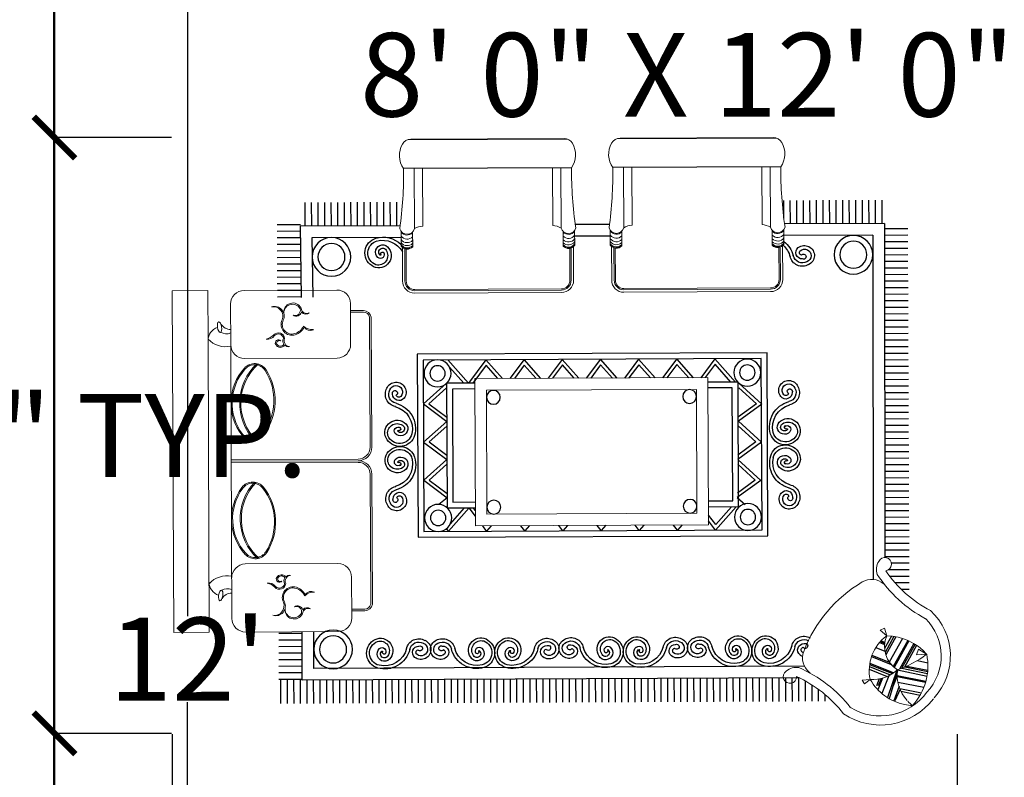
# Model space of a CAD drawing. Units: inches. Extents: x 147 to 1638, y 107 to 941.
# Tile 6 of 17: x 469 to 541, y 315 to 370. Entities that reach past the tile are written whole.
import ezdxf

# ---------------------------------------------------------------- set-up
doc = ezdxf.new("R2010")
doc.units = ezdxf.units.IN
doc.header["$MEASUREMENT"] = 0
for name, color, linetype, lineweight in [('A-ANNO-DIMS', 2, 'Continuous', 15), ('A-AREA-IDEN', 7, 'Continuous', 18), ('furniture', 50, 'Continuous', 18), ('wall', 7, 'Continuous', 60), ('walls', 7, 'Continuous', 50)]:
    doc.layers.add(name, color=color, linetype=linetype, lineweight=lineweight)
doc.layers.add('CARPET', color=40, linetype='Continuous')
doc.styles.get("Standard").update_dxf_attribs({"font": 'arial.ttf'})
doc.dimstyles.get("Standard").update_dxf_attribs({"dimtxt": 6, "dimasz": 3, "dimexe": 0.18, "dimexo": 0.0625, "dimgap": 0.09, "dimtad": 0, "dimtih": 1, "dimtoh": 1, "dimdec": 1, "dimzin": 0, "dimdsep": 46, "dimlunit": 3, "dimtxsty": 'Standard', "dimblk": 'ARCHTICK', "dimcen": 0.09, "dimadec": 0, "dimazin": 0, "dimtfac": 1, "dimtdec": 1, "dimtofl": 0, "dimtmove": 0, "dimatfit": 3, "dimfxl": 1, "dimtolj": 1, "dimtzin": 0, "dimarcsym": 0})

# ---------------------------------------------------------------- blocks, each defined once
blk = doc.blocks.new('_ArchTick')
at = {"color": 0, "linetype": 'ByBlock', "const_width": 0.15}
blk.add_lwpolyline([(-0.5, -0.5), (0.5, 0.5)], dxfattribs=at)
blk = doc.blocks.new('*D28')
at = {"layer": 'A-ANNO-DIMS', "color": 0, "lineweight": -2, "transparency": 16777216}
for p, q in [((483.882, 395.718), (481.394, 395.718)), ((481.574, 395.718), (481.574, 326.82)), ((481.574, 251.718), (481.574, 320.616)), ((483.882, 251.718), (481.394, 251.718))]:
    blk.add_line(p, q, dxfattribs=at)
at = {"layer": 'Defpoints', "color": 0, "lineweight": -2, "transparency": 16777216}
for p in [(483.944, 395.718), (481.574, 251.718), (483.944, 251.718)]:
    blk.add_point(p, dxfattribs=at)
at = {"layer": 'A-ANNO-DIMS', "color": 0, "lineweight": -2, "transparency": 16777216, "xscale": 3, "yscale": 3, "zscale": 3}
for p, rotation in [((481.574, 395.718), 90), ((481.574, 251.718), 270)]:
    blk.add_blockref('_ArchTick', p, dxfattribs=dict(at, rotation=rotation))
at = {"layer": 'A-ANNO-DIMS', "color": 0, "transparency": 16777216, "insert": (481.574, 323.718), "char_height": 6, "attachment_point": 5}
blk.add_mtext("\\A1;12'", dxfattribs=at)
blk = doc.blocks.new('X')
at = {"layer": 'furniture'}
for p, q in [((619.5149, -248.9209), (619.5149, -248.7654)), ((619.5149, -248.7654), (621.0036, -248.7654)), ((621.0036, -248.9205), (621.0036, -248.765)), ((619.5149, -248.9209), (619.7322, -248.9205)), ((619.7322, -248.9205), (620.6015, -248.9205)), ((621.0036, -248.9205), (620.6015, -248.9205)), ((619.5742, -249.0193), (619.752, -249.0193)), ((619.752, -249.0193), (620.6015, -249.0193)), ((620.2516, -249.5725), (620.2516, -249.0193)), ((620.259, -249.5725), (620.259, -249.0193)), ((620.259, -249.5725), (620.259, -249.0193)), ((620.2664, -249.5725), (620.2664, -249.0193)), ((620.9439, -249.0193), (620.6015, -249.0193)), ((619.5149, -249.0786), (619.5149, -249.4824)), ((619.8112, -249.4824), (619.8112, -249.0786)), ((620.7068, -249.4824), (620.7068, -249.0786)), ((621.0032, -249.4824), (621.0032, -249.0786)), ((619.5742, -249.5417), (619.752, -249.5417)), ((619.6049, -249.5417), (619.6049, -249.5987)), ((619.6124, -249.5417), (619.6124, -249.599)), ((620.9439, -249.5417), (620.7661, -249.5417)), ((620.9057, -249.5417), (620.9057, -249.599)), ((620.9131, -249.5417), (620.9131, -249.5987)), ((619.6334, -249.6243), (620.1998, -249.6243)), ((620.8846, -249.6243), (620.3183, -249.6243)), ((619.6334, -249.6317), (620.1998, -249.6317)), ((620.8846, -249.6317), (620.3183, -249.6317))]:
    blk.add_line(p, q, dxfattribs=at)
for centre, radius, start, end in [((619.7322, -248.9798), 0.0593, 90, 162.494), ((619.6556, -248.9979), 0.1044, 348.1465, 47.5301), ((620.8625, -248.9979), 0.1044, 132.4699, 191.8535), ((620.7859, -248.9798), 0.0593, 17.506, 90), ((619.635, -249.0188), 0.0496, 359.4118, 58.4035), ((619.6525, -249.0006), 0.0512, 338.6022, 29.5906), ((620.8656, -249.0006), 0.0512, 150.4094, 201.3978), ((620.8831, -249.0188), 0.0496, 121.5965, 180.5882), ((619.5742, -249.0786), 0.0593, 90, 180), ((619.752, -249.0786), 0.0593, 0, 90), ((620.007, -249.2476), 0.2283, 52.9697, 132.3248), ((620.007, -249.2476), 0.2234, 52.9697, 132.3248), ((620.5111, -249.2476), 0.2283, 47.6752, 127.0303), ((620.5111, -249.2476), 0.2234, 47.6752, 127.0303), ((620.7661, -249.0786), 0.0593, 90, 180), ((620.9439, -249.0786), 0.0593, 0, 90), ((620.007, -249.2904), 0.2333, 46.5317, 137.5727), ((620.007, -249.2904), 0.2283, 45.7406, 138.4308), ((620.1088, -249.1127), 0.0543, 307.9815, 52.9697), ((620.1088, -249.1127), 0.0593, 307.9815, 52.9697), ((620.4092, -249.1127), 0.0593, 127.0303, 232.0185), ((620.5111, -249.2904), 0.2333, 42.4273, 133.4683), ((620.5111, -249.2904), 0.2283, 41.5692, 134.2594), ((620.4092, -249.1127), 0.0543, 127.0303, 232.0185), ((619.8932, -249.1226), 0.0593, 132.3248, 237.3129), ((619.8932, -249.1226), 0.0543, 132.3248, 237.3129), ((620.6249, -249.1226), 0.0543, 302.6871, 47.6752), ((620.6249, -249.1226), 0.0593, 302.6871, 47.6752), ((619.994, -248.9656), 0.241, 237.3129, 307.9815), ((620.5241, -248.9656), 0.241, 232.0185, 302.6871), ((619.6274, -249.2105), 0.0421, 161.9562, 295.8589), ((619.628, -249.2055), 0.0415, 168.8535, 291.9971), ((619.6678, -249.1626), 0.0605, 312.9929, 349.1923), ((619.6905, -249.1804), 0.0373, 306.0062, 9.8559), ((619.994, -248.9656), 0.2459, 237.3129, 307.9815), ((620.5241, -248.9656), 0.2459, 232.0185, 302.6871), ((620.8276, -249.1804), 0.0373, 170.1441, 233.9938), ((620.8503, -249.1626), 0.0605, 190.8077, 227.0071), ((620.8907, -249.2105), 0.0421, 244.1411, 18.0438), ((620.89, -249.2055), 0.0415, 248.0029, 11.1465), ((619.6641, -249.2863), 0.0471, 341.9562, 115.8589), ((619.7278, -249.227), 0.0274, 132.9929, 265.5491), ((619.7278, -249.227), 0.0225, 132.9929, 262.0854), ((619.745, -249.2275), 0.014, 61.3061, 229.1728), ((619.7459, -249.2313), 0.0122, 73.4413, 214.1042), ((619.7406, -249.2356), 0.0182, 302.613, 61.3061), ((619.7406, -249.2356), 0.0232, 306.2825, 61.3061), ((620.7775, -249.2356), 0.0232, 118.6939, 233.7175), ((620.7775, -249.2356), 0.0182, 118.6939, 237.387), ((620.7731, -249.2275), 0.014, 310.8272, 118.6939), ((620.7722, -249.2313), 0.0122, 325.8958, 106.5587), ((620.7903, -249.227), 0.0274, 274.4509, 47.0071), ((620.7903, -249.227), 0.0225, 277.9146, 47.0071), ((620.854, -249.2863), 0.0471, 64.1411, 198.0438), ((619.6105, -249.2907), 0.0399, 81.3465, 244.8004), ((619.6138, -249.2892), 0.0378, 78.8201, 241.2356), ((619.6641, -249.2863), 0.0421, 341.9562, 115.8589), ((619.7361, -249.2716), 0.0251, 55.3181, 117.0875), ((619.7357, -249.2774), 0.0252, 3.6815, 113.5358), ((619.7361, -249.2716), 0.0251, 350.3606, 43.6395), ((620.782, -249.2716), 0.0251, 136.3605, 189.6394), ((620.7824, -249.2774), 0.0252, 66.4642, 176.3185), ((620.782, -249.2716), 0.0251, 62.9125, 124.6819), ((620.854, -249.2863), 0.0421, 64.1411, 198.0438), ((620.9043, -249.2892), 0.0378, 298.7644, 101.1799), ((620.9076, -249.2907), 0.0399, 295.1996, 98.6535), ((619.5921, -249.3513), 0.0246, 333.6734, 86.7751), ((619.6028, -249.3007), 0.0227, 251.5796, 22.4881), ((619.6037, -249.3051), 0.024, 287.888, 33.0148), ((619.5947, -249.3467), 0.0249, 321.2748, 48.9944), ((619.6438, -249.2797), 0.0635, 295.8589, 341.9562), ((619.6438, -249.2797), 0.0684, 298.7765, 341.9562), ((620.8743, -249.2797), 0.0684, 198.0438, 241.2235), ((620.8743, -249.2797), 0.0635, 198.0438, 244.1411), ((620.9144, -249.3051), 0.024, 146.9852, 252.112), ((620.9153, -249.3007), 0.0227, 157.5119, 288.4204), ((620.9233, -249.3467), 0.0249, 131.0056, 218.7252), ((620.926, -249.3513), 0.0246, 93.2249, 206.3266), ((619.6335, -249.3751), 0.0539, 355.2787, 45.2526), ((619.6593, -249.3656), 0.0313, 333.5007, 56.0681), ((620.8588, -249.3656), 0.0313, 123.9319, 206.4993), ((620.8845, -249.3751), 0.0539, 134.7474, 184.7213), ((619.5742, -249.4824), 0.0593, 180, 270), ((619.752, -249.4824), 0.0593, 270, 0), ((620.7661, -249.4824), 0.0593, 180, 270), ((620.9439, -249.4824), 0.0593, 270, 0), ((620.1998, -249.5725), 0.0593, 270, 0), ((620.1998, -249.5725), 0.0519, 270, 0), ((620.3183, -249.5725), 0.0593, 180, 270), ((620.3183, -249.5725), 0.0519, 180, 270), ((619.6387, -249.5984), 0.0338, 180.5447, 260.991), ((619.6384, -249.5987), 0.0261, 179.3782, 258.9715), ((620.8796, -249.5987), 0.0261, 281.0285, 0.6218), ((620.8793, -249.5984), 0.0338, 279.009, 359.4553)]:
    blk.add_arc(centre, radius, start, end, dxfattribs=at)
blk.add_ellipse((619.6743, -248.9709), major_axis=(-0.023, 0.0035), ratio=0.388107, start_param=3.141593, end_param=9.424778, dxfattribs=at)
at = {"layer": 'furniture', "extrusion": (0, 0, -1)}
blk.add_ellipse((620.8437, -248.9709), major_axis=(0.023, 0.0035), ratio=0.388107, start_param=3.141593, end_param=9.424778, dxfattribs=at)
blk = doc.blocks.new('sitting')
at = {"layer": 'CARPET'}
for p, q in [((0.3744, 0.8151), (0.3749, 0.9167)), ((0.403, 0.815), (0.4035, 0.9166)), ((0.4316, 0.8149), (0.432, 0.9165)), ((0.4602, 0.8148), (0.4606, 0.9164)), ((0.4887, 0.8147), (0.4892, 0.9163)), ((0.5173, 0.8145), (0.5178, 0.9161)), ((0.5459, 0.8144), (0.5463, 0.916)), ((0.5745, 0.8143), (0.5749, 0.9159)), ((0.603, 0.8142), (0.6035, 0.9158)), ((0.6316, 0.8141), (0.632, 0.9156)), ((0.6602, 0.8139), (0.6606, 0.9155)), ((0.6888, 0.8138), (0.6892, 0.9154)), ((2.1553, 0.8075), (2.1557, 0.9091)), ((2.1839, 0.8074), (2.1843, 0.909)), ((2.2125, 0.8073), (2.2129, 0.9089)), ((2.241, 0.8072), (2.2415, 0.9088)), ((2.2696, 0.8071), (2.27, 0.9087)), ((2.2982, 0.8069), (2.2986, 0.9085)), ((2.3268, 0.8068), (2.3272, 0.9084)), ((2.3553, 0.8067), (2.3558, 0.9083)), ((2.4602, 0.8713), (2.3589, 0.8717)), ((2.4603, 0.8998), (2.359, 0.9003)), ((2.46, 0.8427), (2.3588, 0.8431)), ((0.3791, 0.7944), (0.2775, 0.7949)), ((0.3793, 0.8151), (0.3774, 0.3798)), ((0.6912, 0.81), (0.3793, 0.8151)), ((0.4301, 0.8149), (0.4301, 0.8143)), ((2.3583, 0.8067), (2.1476, 0.8076)), ((2.349, -1.3602), (2.3583, 0.8067)), ((2.4598, 0.7855), (2.3585, 0.786)), ((2.4599, 0.8141), (2.3586, 0.8145)), ((0.3789, 0.7373), (0.2773, 0.7377)), ((0.379, 0.7658), (0.2774, 0.7663)), ((0.3791, 0.7643), (0.3785, 0.7643)), ((0.4299, 0.7635), (0.4282, 0.3764)), ((0.6904, 0.7592), (0.4299, 0.7635)), ((2.3073, 0.7561), (2.1474, 0.7568)), ((2.2981, -1.3815), (2.3073, 0.7561)), ((2.4597, 0.757), (2.3584, 0.7574)), ((0.3788, 0.7087), (0.2772, 0.7091)), ((2.4594, 0.6998), (2.3582, 0.7002)), ((2.4596, 0.7284), (2.3583, 0.7288)), ((0.3785, 0.6515), (0.2769, 0.652)), ((0.3786, 0.6801), (0.277, 0.6806)), ((2.4593, 0.6712), (2.358, 0.6717)), ((0.3784, 0.623), (0.2768, 0.6234)), ((2.4591, 0.6141), (2.3578, 0.6145)), ((2.4592, 0.6427), (2.3579, 0.6431)), ((0.3782, 0.5658), (0.2766, 0.5663)), ((0.3783, 0.5944), (0.2767, 0.5948)), ((2.4589, 0.5855), (2.3577, 0.586)), ((0.378, 0.5372), (0.2764, 0.5377)), ((2.4587, 0.5284), (2.3574, 0.5288)), ((2.4588, 0.5569), (2.3576, 0.5574)), ((0.3778, 0.4801), (0.2762, 0.4805)), ((0.3779, 0.5087), (0.2763, 0.5091)), ((2.4586, 0.4998), (2.3573, 0.5002)), ((0.3777, 0.4515), (0.2761, 0.452)), ((2.4583, 0.4426), (2.3571, 0.4431)), ((2.4585, 0.4712), (2.3572, 0.4717)), ((0.3774, 0.3944), (0.2758, 0.3948)), ((0.3775, 0.4229), (0.2759, 0.4234)), ((2.4582, 0.4141), (2.3569, 0.4145)), ((2.458, 0.3569), (2.3567, 0.3574)), ((2.4581, 0.3855), (2.3568, 0.3859)), ((2.4578, 0.3283), (2.3566, 0.3288)), ((1.065, 0.178), (1.1552, 0.2792)), ((1.1552, 0.2792), (1.2313, 0.1773)), ((1.2313, 0.1773), (1.3215, 0.2785)), ((1.3215, 0.2785), (1.3976, 0.1766)), ((1.3976, 0.1766), (1.4877, 0.2778)), ((1.4877, 0.2778), (1.5638, 0.1759)), ((2.4576, 0.2712), (2.3563, 0.2716)), ((2.4577, 0.2998), (2.3565, 0.3002)), ((1.0854, 0.1779), (1.1542, 0.2552)), ((1.1542, 0.2552), (1.2122, 0.1774)), ((1.2516, 0.1772), (1.3204, 0.2544)), ((1.3204, 0.2544), (1.3785, 0.1767)), ((1.4179, 0.1765), (1.4867, 0.2537)), ((1.4867, 0.2537), (1.5447, 0.176)), ((2.4575, 0.2426), (2.3562, 0.2431)), ((1.0646, 0.0827), (0.9634, 0.1728)), ((1.5638, 0.1759), (1.5928, 0.2111)), ((1.7096, 0.1696), (1.6979, 0.1786)), ((2.4572, 0.1855), (2.356, 0.1859)), ((2.4574, 0.214), (2.3561, 0.2145)), ((1.0647, 0.103), (0.9951, 0.165)), ((1.6077, 0.0803), (1.7096, 0.1696)), ((1.6077, 0.1007), (1.6779, 0.1621)), ((2.457, 0.1283), (2.3557, 0.1288)), ((2.4571, 0.1569), (2.3558, 0.1573)), ((2.4569, 0.0997), (2.3556, 0.1002)), ((0.9627, 0.0066), (1.0646, 0.0827)), ((0.9868, 0.0055), (1.0646, 0.0636)), ((1.6188, 0.0528), (1.6076, 0.0613)), ((1.6441, 0.0527), (1.6077, 0.0803)), ((2.4566, 0.0426), (2.3554, 0.043)), ((2.4567, 0.0712), (2.3555, 0.0716)), ((1.0444, -0.0662), (0.9627, 0.0066)), ((1.0444, -0.0458), (0.9868, 0.0055)), ((1.6859, -0.0168), (1.7089, 0.0034)), ((1.7089, 0.0034), (1.6861, 0.0207)), ((2.4565, 0.014), (2.3552, 0.0145)), ((2.4563, -0.0431), (2.355, -0.0427)), ((2.4564, -0.0146), (2.3551, -0.0141)), ((2.4561, -0.0717), (2.3549, -0.0713)), ((0.962, -0.1597), (1.0442, -0.0983)), ((0.9861, -0.1607), (1.0441, -0.1174)), ((2.4559, -0.1288), (2.3546, -0.1284)), ((2.456, -0.1003), (2.3547, -0.0998)), ((1.0436, -0.2324), (0.962, -0.1597)), ((1.0437, -0.2121), (0.9861, -0.1607)), ((1.6852, -0.183), (1.7082, -0.1629)), ((1.7082, -0.1629), (1.6854, -0.1455)), ((2.4558, -0.1574), (2.3545, -0.157)), ((2.4555, -0.2146), (2.3543, -0.2141)), ((2.4557, -0.186), (2.3544, -0.1856)), ((2.4554, -0.2431), (2.3541, -0.2427)), ((0.9613, -0.326), (1.0435, -0.2646)), ((0.9854, -0.327), (1.0434, -0.2837)), ((2.4552, -0.3003), (2.3539, -0.2999)), ((2.4553, -0.2717), (2.354, -0.2713)), ((1.0429, -0.3987), (0.9613, -0.326)), ((1.043, -0.3784), (0.9854, -0.327)), ((1.6845, -0.3493), (1.7075, -0.3291)), ((1.7075, -0.3291), (1.6847, -0.3118)), ((2.455, -0.3289), (2.3538, -0.3284)), ((0.3734, -0.5318), (0.374, -0.383)), ((0.4242, -0.5353), (0.4248, -0.38)), ((2.4548, -0.386), (2.3535, -0.3856)), ((2.4549, -0.3574), (2.3537, -0.357)), ((2.4547, -0.4146), (2.3534, -0.4142)), ((0.9606, -0.4922), (1.0428, -0.4308)), ((0.9847, -0.4933), (1.0427, -0.4499)), ((2.4544, -0.4717), (2.3532, -0.4713)), ((2.4546, -0.4432), (2.3533, -0.4427)), ((1.0422, -0.5649), (0.9606, -0.4922)), ((1.0423, -0.5446), (0.9847, -0.4933)), ((1.6838, -0.5155), (1.7068, -0.4954)), ((1.7068, -0.4954), (1.684, -0.478)), ((2.4543, -0.5003), (2.353, -0.4999)), ((2.4541, -0.5575), (2.3528, -0.557)), ((2.4542, -0.5289), (2.3529, -0.5285)), ((0.9599, -0.6585), (1.0421, -0.5971)), ((2.4539, -0.586), (2.3527, -0.5856)), ((0.984, -0.6595), (1.042, -0.6162)), ((2.4537, -0.6432), (2.3524, -0.6428)), ((2.4538, -0.6146), (2.3526, -0.6142)), ((1.0415, -0.7312), (0.9599, -0.6585)), ((1.0416, -0.7109), (0.984, -0.6595)), ((1.6831, -0.6818), (1.7061, -0.6617)), ((1.7061, -0.6617), (1.6833, -0.6443)), ((2.4536, -0.6718), (2.3523, -0.6713)), ((2.4533, -0.7289), (2.3521, -0.7285)), ((2.4535, -0.7003), (2.3522, -0.6999)), ((0.9592, -0.8247), (1.0414, -0.7634)), ((2.4532, -0.7575), (2.3519, -0.7571)), ((0.9832, -0.8258), (1.0413, -0.7824)), ((1.7054, -0.8279), (1.6825, -0.8106)), ((2.453, -0.8146), (2.3517, -0.8142)), ((2.4531, -0.7861), (2.3518, -0.7856)), ((1.0408, -0.8975), (0.9592, -0.8247)), ((1.0409, -0.8771), (0.9832, -0.8258)), ((1.6824, -0.8481), (1.7054, -0.8279)), ((2.4528, -0.8432), (2.3516, -0.8428)), ((2.4526, -0.9004), (2.3513, -0.8999)), ((2.4527, -0.8718), (2.3515, -0.8714)), ((0.9585, -0.991), (1.0407, -0.9296)), ((2.4525, -0.9289), (2.3512, -0.9285)), ((0.9825, -0.992), (1.0406, -0.9487)), ((1.6806, -0.995), (1.6392, -0.9636)), ((1.7047, -0.9942), (1.6645, -0.9637)), ((2.4522, -0.9861), (2.351, -0.9857)), ((2.4524, -0.9575), (2.3511, -0.9571)), ((1.0597, -1.0812), (0.9585, -0.991)), ((1.0598, -1.0608), (0.9825, -0.992)), ((1.6027, -1.0835), (1.7047, -0.9942)), ((1.6028, -1.0632), (1.6806, -0.995)), ((2.4521, -1.0147), (2.3508, -1.0142)), ((2.4519, -1.0718), (2.3506, -1.0714)), ((2.452, -1.0432), (2.3507, -1.0428)), ((1.0645, -1.0959), (1.1557, -1.1962)), ((1.0848, -1.0956), (1.1544, -1.1721)), ((1.1544, -1.1721), (1.2117, -1.0938)), ((1.1557, -1.1962), (1.2307, -1.0935)), ((1.2307, -1.0935), (1.3219, -1.1938)), ((1.2511, -1.0932), (1.3206, -1.1697)), ((1.3206, -1.1697), (1.3779, -1.0914)), ((1.3219, -1.1938), (1.397, -1.0911)), ((1.397, -1.0911), (1.4882, -1.1914)), ((1.4173, -1.0908), (1.4869, -1.1674)), ((1.4869, -1.1674), (1.5442, -1.089)), ((1.4882, -1.1914), (1.5632, -1.0887)), ((1.5632, -1.0887), (1.5926, -1.1237)), ((2.4517, -1.1004), (2.3505, -1.1)), ((2.4515, -1.1575), (2.3502, -1.1571)), ((2.4516, -1.129), (2.3504, -1.1285)), ((2.4514, -1.1861), (2.3501, -1.1857)), ((2.4511, -1.2433), (2.3499, -1.2428)), ((2.4513, -1.2147), (2.35, -1.2143)), ((2.451, -1.2718), (2.3498, -1.2714)), ((0.3701, -1.3201), (0.2685, -1.3197)), ((0.3458, -1.2914), (0.2686, -1.2911)), ((0.3684, -1.73), (0.3702, -1.2947)), ((0.4194, -1.6792), (0.421, -1.2917)), ((2.4508, -1.329), (2.3495, -1.3286)), ((2.4509, -1.3004), (2.3496, -1.3)), ((0.37, -1.3487), (0.2684, -1.3483)), ((2.4507, -1.3576), (2.3494, -1.3571)), ((0.3697, -1.4058), (0.2681, -1.4054)), ((0.3699, -1.3773), (0.2683, -1.3768)), ((2.4505, -1.3861), (2.3623, -1.3858)), ((2.4504, -1.4147), (2.3793, -1.4144)), ((0.3696, -1.4344), (0.268, -1.434)), ((2.4503, -1.4433), (2.3989, -1.4431)), ((0.3694, -1.4916), (0.2678, -1.4911)), ((0.3695, -1.463), (0.2679, -1.4626)), ((2.4502, -1.4719), (2.4215, -1.4717)), ((0.3693, -1.5201), (0.2677, -1.5197)), ((0.369, -1.5773), (0.2674, -1.5769)), ((0.3691, -1.5487), (0.2675, -1.5483)), ((0.3689, -1.6059), (0.2673, -1.6054)), ((0.3686, -1.663), (0.267, -1.6626)), ((0.3688, -1.6344), (0.2672, -1.634)), ((2.2845, -1.6663), (2.3262, -1.7708)), ((2.2896, -1.6655), (2.3296, -1.7657)), ((2.2995, -1.6644), (2.3358, -1.7553)), ((2.3112, -1.6637), (2.3424, -1.7417)), ((0.3685, -1.6916), (0.2669, -1.6912)), ((0.3685, -1.6792), (0.3686, -1.6792)), ((0.4194, -1.6792), (1.9199, -1.6809)), ((2.1869, -1.7158), (2.1934, -1.732)), ((2.1905, -1.7124), (2.1981, -1.7313)), ((2.1949, -1.7086), (2.2037, -1.7307)), ((2.2165, -1.6925), (2.2322, -1.7319)), ((2.2497, -1.6758), (2.2797, -1.7508)), ((2.2561, -1.6735), (2.2901, -1.7588)), ((2.3496, -1.7218), (2.4007, -1.7017)), ((2.3514, -1.7152), (2.3825, -1.7029)), ((2.353, -1.7075), (2.3836, -1.6955)), ((0.3684, -1.7202), (0.2668, -1.7197)), ((0.3684, -1.73), (1.8242, -1.7316)), ((0.3917, -1.8317), (0.3922, -1.7301)), ((0.4203, -1.8318), (0.4207, -1.7302)), ((0.4489, -1.8319), (0.4493, -1.7303)), ((0.4775, -1.832), (0.4779, -1.7304)), ((0.506, -1.8322), (0.5065, -1.7306)), ((0.5346, -1.8323), (0.535, -1.7307)), ((0.5632, -1.8324), (0.5636, -1.7308)), ((0.5917, -1.8325), (0.5922, -1.7309)), ((0.6203, -1.8327), (0.6208, -1.7311)), ((0.6489, -1.8328), (0.6493, -1.7312)), ((0.6775, -1.8329), (0.6779, -1.7313)), ((0.6775, -1.8329), (0.6779, -1.7313)), ((0.706, -1.833), (0.7065, -1.7314)), ((0.7346, -1.8331), (0.7351, -1.7315)), ((0.7632, -1.8333), (0.7636, -1.7317)), ((0.7918, -1.8334), (0.7922, -1.7318)), ((0.8203, -1.8335), (0.8208, -1.7319)), ((0.8489, -1.8336), (0.8494, -1.732)), ((0.8775, -1.8338), (0.8779, -1.7322)), ((0.9061, -1.8339), (0.9065, -1.7323)), ((0.9346, -1.834), (0.9351, -1.7324)), ((0.9632, -1.8341), (0.9637, -1.7325)), ((0.9632, -1.8341), (0.9637, -1.7325)), ((0.9918, -1.8342), (0.9922, -1.7326)), ((1.0204, -1.8344), (1.0208, -1.7328)), ((1.0489, -1.8345), (1.0494, -1.7329)), ((1.0775, -1.8346), (1.078, -1.733)), ((1.1061, -1.8347), (1.1065, -1.7331)), ((1.1347, -1.8349), (1.1351, -1.7333)), ((1.1632, -1.835), (1.1637, -1.7334)), ((1.1918, -1.8351), (1.1923, -1.7335)), ((1.2204, -1.8352), (1.2208, -1.7336)), ((1.249, -1.8353), (1.2494, -1.7337)), ((1.249, -1.8353), (1.2494, -1.7337)), ((1.2775, -1.8355), (1.278, -1.7339)), ((1.3061, -1.8356), (1.3066, -1.734)), ((1.3347, -1.8357), (1.3351, -1.7341)), ((1.3633, -1.8358), (1.3637, -1.7342)), ((1.3918, -1.8359), (1.3923, -1.7344)), ((1.4204, -1.8361), (1.4209, -1.7345)), ((1.449, -1.8362), (1.4494, -1.7346)), ((1.4776, -1.8363), (1.478, -1.7347)), ((1.5061, -1.8364), (1.5066, -1.7348)), ((1.5347, -1.8366), (1.5351, -1.735)), ((1.5347, -1.8366), (1.5351, -1.735)), ((1.5633, -1.8367), (1.5637, -1.7351)), ((1.5919, -1.8368), (1.5923, -1.7352)), ((1.6204, -1.8369), (1.6209, -1.7353)), ((1.649, -1.837), (1.6494, -1.7354)), ((1.6776, -1.8372), (1.678, -1.7356)), ((1.7062, -1.8373), (1.7066, -1.7357)), ((1.7347, -1.8374), (1.7352, -1.7358)), ((1.7633, -1.8375), (1.7637, -1.7359)), ((1.7919, -1.8377), (1.7923, -1.7361)), ((1.8205, -1.8378), (1.8209, -1.7362)), ((1.8205, -1.8378), (1.8209, -1.7362)), ((1.8776, -1.838), (1.878, -1.7463)), ((1.9062, -1.8381), (1.9065, -1.7539)), ((2.1669, -1.7607), (2.2209, -1.7306)), ((2.1682, -1.7716), (2.2377, -1.7329)), ((2.1696, -1.7798), (2.2486, -1.7358)), ((2.1767, -1.8083), (2.2798, -1.7509)), ((2.3154, -1.7846), (2.4341, -1.7427)), ((2.3177, -1.7875), (2.4393, -1.7513)), ((2.3392, -1.7487), (2.4162, -1.7184)), ((1.849, -1.8379), (1.8494, -1.7604)), ((1.9348, -1.8383), (1.935, -1.7772)), ((1.9348, -1.8383), (1.935, -1.7772)), ((2.1854, -1.8315), (2.2996, -1.7679)), ((2.1876, -1.8364), (2.3032, -1.7719)), ((2.1988, -1.8576), (2.3106, -1.7953)), ((2.3142, -1.7864), (2.3404, -1.9165)), ((2.3375, -1.7853), (2.3628, -1.9109)), ((2.3403, -1.7854), (2.3836, -1.7684)), ((2.3425, -1.7855), (2.3676, -1.9096)), ((2.3667, -1.7885), (2.3896, -1.9022)), ((2.3849, -1.7941), (2.4485, -1.7704)), ((2.3952, -1.797), (2.4141, -1.8911)), ((2.3975, -1.7979), (2.448, -1.7755)), ((2.4068, -1.802), (2.4237, -1.8859)), ((1.9633, -1.8384), (1.9635, -1.8042)), ((2.2023, -1.8633), (2.3072, -1.8049)), ((2.2069, -1.8702), (2.3018, -1.8173)), ((2.297, -1.8281), (2.3153, -1.9188)), ((2.3011, -1.8189), (2.3211, -1.9184)), ((2.3067, -1.8053), (2.3293, -1.9175)), ((2.2731, -1.8735), (2.2823, -1.919))]:
    blk.add_line(p, q, dxfattribs=at)
for points in [[(0.9321, -1.2188), (0.9386, 0.3056), (1.7356, 0.3022), (1.7291, -1.2222)], [(0.9576, -1.1935), (0.9639, 0.2801), (1.7101, 0.2769), (1.7038, -1.1967)]]:
    blk.add_lwpolyline(points, close=True, dxfattribs=at)
for points in [[(1.0645, 0.0551), (1.065, 0.178), (1.6081, 0.1757), (1.6075, 0.0528)], [(1.0899, 0.055), (1.0903, 0.1525), (1.5826, 0.1504), (1.5821, 0.0529)], [(1.6032, -0.9634), (1.6026, -1.0947), (1.0596, -1.0923), (1.0602, -0.9611)], [(1.5778, -0.9633), (1.5774, -1.0692), (1.0851, -1.0671), (1.0856, -0.9612)]]:
    blk.add_lwpolyline(points, dxfattribs=at)
for centre, radius in [((0.5147, 0.6796), 0.0843), ((0.5147, 0.6796), 0.0589), ((2.2246, 0.6725), 0.0843), ((2.2246, 0.6725), 0.0589), ((1.022, 0.2174), 0.0589), ((1.6516, 0.2147), 0.0589), ((1.022, 0.2174), 0.0335), ((1.6516, 0.2147), 0.0335), ((1.1262, -0.0259), 0.0301), ((1.6047, -0.028), 0.0301), ((1.1225, -0.881), 0.0301), ((1.601, -0.883), 0.0301), ((1.0184, -1.1325), 0.0589), ((1.0184, -1.1325), 0.0335), ((1.6479, -1.1352), 0.0589), ((1.6479, -1.1352), 0.0335), ((0.505, -1.5948), 0.0843), ((0.505, -1.5948), 0.0589)]:
    blk.add_circle(centre, radius, dxfattribs=at)
for centre, radius, start, end in [((0.497, 0.4669), 0.067, 33.9233, 162.7475), ((0.4977, 0.4665), 0.0548, 20.9066, 165.9288), ((2.2413, 0.4595), 0.067, 16.7636, 145.5879), ((0.5416, 0.4551), 0.1132, 163.7275, 224.1633), ((0.5428, 0.4571), 0.1008, 166.9963, 238.9602), ((0.4936, 0.4564), 0.0315, 41.0431, 239.8965), ((0.4936, 0.4564), 0.0169, 41.0431, 239.8965), ((0.5086, 0.4733), 0.0538, 235.0798, 35.1804), ((0.5086, 0.4759), 0.0415, 235.3613, 14.077), ((0.5048, 0.4662), 0.0166, 231.0878, 41.0431), ((2.2298, 0.466), 0.0538, 144.3308, 304.4313), ((2.2297, 0.4686), 0.0415, 165.4341, 304.1498), ((2.2406, 0.459), 0.0548, 13.5823, 158.6045), ((2.2447, 0.449), 0.0315, 299.6146, 138.468), ((2.1966, 0.448), 0.1132, 284.4505, 15.7836), ((0.5005, 0.4578), 0.00755, 65.8585, 269.2935), ((0.5048, 0.4662), 0.00198, 231.0878, 41.0431), ((1.1039, 0.3982), 0.0436, 112.8813, 307.2162), ((1.1129, 0.3899), 0.055, 11.9905, 119.1807), ((1.1129, 0.3899), 0.0404, 11.9905, 119.1807), ((1.2799, 0.3933), 0.0538, 54.3308, 214.4313), ((1.2825, 0.3934), 0.0415, 75.4341, 214.1498), ((1.273, 0.3825), 0.0548, 283.5823, 68.6045), ((1.2734, 0.3818), 0.067, 286.7636, 55.5879), ((1.4074, 0.3811), 0.067, 123.9233, 252.7475), ((1.4078, 0.3819), 0.0548, 110.9066, 255.9288), ((1.401, 0.3927), 0.0538, 325.0798, 125.1804), ((1.3984, 0.3928), 0.0415, 325.3613, 104.077), ((1.5679, 0.3879), 0.055, 60.3304, 167.5206), ((1.577, 0.3961), 0.0436, 232.2949, 66.6298), ((2.2335, 0.4588), 0.0166, 138.468, 308.4233), ((2.1954, 0.45), 0.1008, 284.1961, 12.5148), ((2.2335, 0.4588), 0.00198, 138.468, 308.4233), ((2.2447, 0.449), 0.0169, 299.6146, 138.468), ((2.2377, 0.4504), 0.00755, 270.2176, 113.6526), ((1.1031, 0.3985), 0.0284, 110.3248, 311.5308), ((1.1077, 0.403), 0.011, 65.5074, 327.1174), ((1.1131, 0.3853), 0.0277, 308.2602, 91.7304), ((1.1133, 0.3856), 0.012, 316.0094, 72.4481), ((1.262, 0.4266), 0.1132, 194.4505, 285.7836), ((1.264, 0.4277), 0.1008, 194.1961, 282.5148), ((1.2629, 0.3785), 0.0315, 209.6146, 48.468), ((1.2629, 0.3785), 0.0169, 209.6146, 48.468), ((1.2728, 0.3896), 0.0166, 48.468, 218.4233), ((1.2643, 0.3854), 0.00755, 180.2176, 23.6526), ((1.2728, 0.3896), 0.00198, 48.468, 218.4233), ((1.4179, 0.3777), 0.0315, 131.0431, 329.8965), ((1.4192, 0.4258), 0.1132, 253.7275, 345.0606), ((1.4172, 0.4269), 0.1008, 256.9963, 345.315), ((1.4081, 0.389), 0.0166, 321.0878, 131.0431), ((1.4179, 0.3777), 0.0169, 131.0431, 329.8965), ((1.4081, 0.389), 0.00198, 321.0878, 131.0431), ((1.4165, 0.3846), 0.00755, 155.8585, 359.2935), ((1.5679, 0.3879), 0.0404, 60.3304, 167.5206), ((1.5677, 0.3833), 0.0277, 87.7807, 231.2509), ((1.5675, 0.3835), 0.012, 107.063, 223.5017), ((1.5778, 0.3964), 0.0284, 227.9804, 69.1863), ((1.5733, 0.4009), 0.011, 212.3938, 114.0037), ((2.2332, 0.299), 0.055, 101.9905, 209.1807), ((2.2249, 0.29), 0.0436, 202.8813, 37.2162), ((2.2332, 0.299), 0.0404, 101.9905, 209.1807), ((2.2246, 0.2892), 0.0284, 200.3248, 41.5308), ((2.2201, 0.2937), 0.011, 155.5074, 57.1174), ((2.2378, 0.2991), 0.0277, 38.2602, 181.7304), ((2.2376, 0.2994), 0.012, 46.0094, 162.4481), ((2.2327, 0.1959), 0.055, 150.3304, 257.5206), ((2.2245, 0.205), 0.0436, 322.2949, 156.6298), ((2.2327, 0.1959), 0.0404, 150.3304, 257.5206), ((2.2243, 0.2058), 0.0284, 317.9804, 159.1863), ((2.2197, 0.2012), 0.011, 302.3938, 204.0037), ((2.2374, 0.1957), 0.0277, 177.7807, 321.2509), ((2.2371, 0.1955), 0.012, 197.063, 313.5017), ((2.1937, 0.0451), 0.1008, 346.9963, 75.315), ((2.1948, 0.0472), 0.1132, 343.7275, 75.0606), ((2.2279, 0.0289), 0.0538, 55.0798, 215.1804), ((2.2278, 0.0263), 0.0415, 55.3613, 194.077), ((2.2317, 0.036), 0.0166, 51.0878, 221.0431), ((2.2429, 0.0458), 0.0315, 221.0431, 59.8965), ((2.2429, 0.0458), 0.0169, 221.0431, 59.8965), ((2.236, 0.0445), 0.00755, 245.8585, 89.2935), ((2.2395, 0.0353), 0.067, 213.9233, 342.7475), ((2.2388, 0.0358), 0.0548, 200.9066, 345.9288), ((2.2317, 0.036), 0.00198, 51.0878, 221.0431), ((2.239, -0.0986), 0.067, 16.7636, 145.5879), ((2.2275, -0.0922), 0.0538, 144.3308, 304.4313), ((2.2274, -0.0895), 0.0415, 165.4341, 304.1498), ((2.2383, -0.0991), 0.0548, 13.5823, 158.6045), ((2.2424, -0.1091), 0.0315, 299.6146, 138.468), ((2.1942, -0.1101), 0.1132, 284.4505, 15.7836), ((2.2312, -0.0993), 0.0166, 138.468, 308.4233), ((2.1931, -0.1081), 0.1008, 284.1961, 12.5148), ((2.2312, -0.0993), 0.00198, 138.468, 308.4233), ((2.2424, -0.1091), 0.0169, 299.6146, 138.468), ((2.2354, -0.1077), 0.00755, 270.2176, 113.6526), ((2.2309, -0.2591), 0.055, 101.9905, 209.1807), ((2.2226, -0.2681), 0.0436, 202.8813, 37.2162), ((2.2309, -0.2591), 0.0404, 101.9905, 209.1807), ((2.2223, -0.2689), 0.0284, 200.3248, 41.5308), ((2.2178, -0.2644), 0.011, 155.5074, 57.1174), ((2.2355, -0.259), 0.0277, 38.2602, 181.7304), ((2.2352, -0.2587), 0.012, 46.0094, 162.4481), ((2.2282, -0.3643), 0.055, 150.3304, 257.5206), ((2.22, -0.3553), 0.0436, 322.2949, 156.6298), ((2.2197, -0.3545), 0.0284, 317.9804, 159.1863), ((2.2282, -0.3643), 0.0404, 150.3304, 257.5206), ((2.2152, -0.359), 0.011, 302.3938, 204.0037), ((2.2328, -0.3646), 0.0277, 177.7807, 321.2509), ((2.2326, -0.3648), 0.012, 197.063, 313.5017), ((2.1892, -0.5151), 0.1008, 346.9963, 75.315), ((2.1903, -0.5131), 0.1132, 343.7275, 75.0606), ((2.2234, -0.5313), 0.0538, 55.0798, 215.1804), ((2.2233, -0.5339), 0.0415, 55.3613, 194.077), ((2.2276, -0.5255), 0.0166, 51.0878, 221.0431), ((2.2384, -0.5144), 0.0315, 221.0431, 59.8965), ((2.2384, -0.5144), 0.0169, 221.0431, 59.8965), ((2.232, -0.5171), 0.00755, 245.8585, 89.2935), ((2.235, -0.5249), 0.067, 213.9233, 342.7475), ((2.2342, -0.5244), 0.0548, 200.9066, 345.9288), ((2.2276, -0.5255), 0.00198, 51.0878, 221.0431), ((2.2345, -0.6588), 0.067, 16.7636, 145.5879), ((2.2229, -0.6524), 0.0538, 144.3308, 304.4313), ((2.2229, -0.6498), 0.0415, 165.4341, 304.1498), ((2.2337, -0.6593), 0.0548, 13.5823, 158.6045), ((2.2378, -0.6694), 0.0315, 299.6146, 138.468), ((2.1897, -0.6703), 0.1132, 284.4505, 15.7836), ((2.2271, -0.6608), 0.0166, 138.468, 308.4233), ((2.1886, -0.6683), 0.1008, 284.1961, 12.5148), ((2.2378, -0.6694), 0.0169, 299.6146, 138.468), ((2.2271, -0.6608), 0.00198, 138.468, 308.4233), ((2.2314, -0.6693), 0.00755, 270.2176, 113.6526), ((2.2263, -0.8194), 0.055, 101.9905, 209.1807), ((2.218, -0.8284), 0.0436, 202.8813, 37.2162), ((2.2263, -0.8194), 0.0404, 101.9905, 209.1807), ((2.2177, -0.8292), 0.0284, 200.3248, 41.5308), ((2.2309, -0.8192), 0.0277, 38.2602, 181.7304), ((2.2307, -0.819), 0.012, 46.0094, 162.4481), ((2.2132, -0.8246), 0.011, 155.5074, 57.1174), ((2.2242, -0.9246), 0.055, 150.3304, 257.5206), ((2.216, -0.9155), 0.0436, 322.2949, 156.6298), ((2.2157, -0.9147), 0.0284, 317.9804, 159.1863), ((2.2242, -0.9246), 0.0404, 150.3304, 257.5206), ((2.2112, -0.9192), 0.011, 302.3938, 204.0037), ((2.2288, -0.9248), 0.0277, 177.7807, 321.2509), ((2.2286, -0.925), 0.012, 197.063, 313.5017), ((2.1852, -1.0753), 0.1008, 346.9963, 75.315), ((2.1863, -1.0733), 0.1132, 343.7275, 75.0606), ((2.2194, -1.0915), 0.0538, 55.0798, 215.1804), ((2.2193, -1.0941), 0.0415, 55.3613, 194.077), ((2.2231, -1.0844), 0.0166, 51.0878, 221.0431), ((2.2344, -1.0746), 0.0315, 221.0431, 59.8965), ((2.2344, -1.0746), 0.0169, 221.0431, 59.8965), ((2.2275, -1.076), 0.00755, 245.8585, 89.2935), ((2.231, -1.0852), 0.067, 213.9233, 342.7475), ((2.2302, -1.0847), 0.0548, 200.9066, 345.9288), ((2.2231, -1.0844), 0.00198, 51.0878, 221.0431), ((2.2305, -1.2191), 0.067, 16.7636, 145.5879), ((2.2189, -1.2126), 0.0538, 144.3308, 304.4313), ((2.2189, -1.21), 0.0415, 165.4341, 304.1498), ((2.2297, -1.2195), 0.0548, 13.5823, 158.6045), ((2.2338, -1.2296), 0.0315, 299.6146, 138.468), ((2.1857, -1.2305), 0.1132, 284.4505, 15.7836), ((1.2544, -1.3426), 0.1132, 73.7275, 165.0606), ((1.2564, -1.3437), 0.1008, 76.9963, 165.315), ((1.2663, -1.2979), 0.067, 303.9233, 72.7475), ((1.4002, -1.2984), 0.067, 106.7636, 235.5879), ((1.4117, -1.3432), 0.1132, 14.4505, 105.7836), ((1.4096, -1.3443), 0.1008, 14.1961, 102.5148), ((2.2231, -1.221), 0.0166, 138.468, 308.4233), ((2.1846, -1.2285), 0.1008, 284.1961, 12.5148), ((2.2338, -1.2296), 0.0169, 299.6146, 138.468), ((2.2231, -1.221), 0.00198, 138.468, 308.4233), ((2.2274, -1.2295), 0.00755, 270.2176, 113.6526), ((1.0966, -1.3129), 0.0436, 52.2949, 246.6298), ((1.0958, -1.3131), 0.0284, 47.9804, 249.1863), ((1.1059, -1.3), 0.0277, 267.7807, 51.2509), ((1.2726, -1.3095), 0.0538, 145.0798, 305.1804), ((1.2558, -1.2945), 0.0315, 311.0431, 149.8965), ((1.2753, -1.3096), 0.0415, 145.3613, 284.077), ((1.2558, -1.2945), 0.0169, 311.0431, 149.8965), ((1.2658, -1.2986), 0.0548, 290.9066, 75.9288), ((1.4007, -1.2991), 0.0548, 103.5823, 248.6045), ((1.3937, -1.3099), 0.0538, 234.3308, 34.4313), ((1.4107, -1.295), 0.0315, 29.6146, 228.468), ((1.3911, -1.31), 0.0415, 255.4341, 34.1498), ((1.4107, -1.295), 0.0169, 29.6146, 228.468), ((1.5605, -1.3019), 0.0277, 128.2602, 271.7304), ((1.5697, -1.3148), 0.0436, 292.8813, 127.2162), ((1.5705, -1.3151), 0.0284, 290.3248, 131.5308), ((0.5381, -1.2235), 0.1132, 217.1139, 255.0606), ((0.5393, -1.2215), 0.1008, 221.6767, 255.315), ((0.5002, -1.3723), 0.055, 330.3304, 77.5206), ((1.1057, -1.3047), 0.055, 240.3304, 347.5206), ((1.1057, -1.3047), 0.0404, 240.3304, 347.5206), ((1.1003, -1.3177), 0.011, 32.3938, 294.0037), ((1.1061, -1.3003), 0.012, 287.063, 43.5017), ((1.2656, -1.3057), 0.0166, 141.0878, 311.0431), ((1.2571, -1.3014), 0.00755, 335.8585, 179.2935), ((1.2656, -1.3057), 0.00198, 141.0878, 311.0431), ((1.4008, -1.3062), 0.0166, 228.468, 38.4233), ((1.4008, -1.3062), 0.00198, 228.468, 38.4233), ((1.4093, -1.302), 0.00755, 0.2176, 203.6526), ((1.5607, -1.3065), 0.055, 191.9905, 299.1807), ((1.5607, -1.3065), 0.0404, 191.9905, 299.1807), ((1.5603, -1.3022), 0.012, 136.0094, 252.4481), ((1.5659, -1.3196), 0.011, 245.5074, 147.1174), ((2.2223, -1.3796), 0.055, 101.9905, 209.1807), ((0.5085, -1.3813), 0.0436, 142.2949, 336.6298), ((0.4956, -1.372), 0.0277, 357.7807, 141.2509), ((0.5087, -1.3821), 0.0284, 137.9804, 339.1863), ((0.4959, -1.3718), 0.012, 17.063, 133.5017), ((0.5133, -1.3776), 0.011, 122.3938, 24.0037), ((0.5002, -1.3723), 0.0404, 330.3304, 77.5206), ((2.2223, -1.3796), 0.0404, 101.9905, 209.1807), ((2.2269, -1.3794), 0.0277, 38.2602, 181.7304), ((2.2267, -1.3792), 0.012, 46.0094, 162.4481), ((2.2137, -1.3894), 0.0284, 26.9755, 41.5308), ((2.214, -1.3886), 0.0436, 20.3174, 37.2162), ((2.2092, -1.3848), 0.011, 155.5074, 57.1174)]:
    blk.add_arc(centre, radius, start, end, dxfattribs=at)
at = {"layer": 'furniture'}
for p, q in [((0.0011, -0.3483), (0.0041, 0.3483)), ((0.1243, -0.3679), (0.1274, 0.3668)), ((0.1263, -0.3665), (0.1294, 0.3654)), ((0.4025, 0.3765), (0.4672, 0.3762)), ((0.473, 0.3708), (0.6194, 0.3702)), ((0.4789, 0.3601), (0.6193, 0.3595)), ((0.4802, 0.3548), (0.6193, 0.3542)), ((-0.0014, -0.3337), (0.0014, 0.3337)), ((0.1292, 0.319), (0.3914, 0.3179)), ((0.4057, 0.326), (0.4705, 0.3258)), ((0.6537, -0.3223), (0.6564, 0.3168)), ((0.659, -0.3224), (0.6618, 0.3167)), ((0.6697, -0.3224), (0.6724, 0.3167)), ((0.129, 0.2827), (0.3801, 0.2816)), ((1.0405, -0.961), (1.0449, 0.0552)), ((1.0449, 0.0552), (1.6862, 0.0525)), ((1.6862, 0.0525), (1.6819, -0.9637)), ((1.0916, -0.9104), (1.0955, 0.0042)), ((1.0955, 0.0042), (1.6352, 0.0019)), ((1.6352, 0.0019), (1.6313, -0.9127)), ((0.1266, -0.2838), (0.3777, -0.2849)), ((0.1265, -0.3201), (0.3887, -0.3212)), ((0.4029, -0.3295), (0.4677, -0.3298)), ((0.3992, -0.3799), (0.464, -0.3802)), ((0.4698, -0.3748), (0.6162, -0.3754)), ((0.4758, -0.3642), (0.6162, -0.3648)), ((0.4772, -0.3589), (0.6163, -0.3595)), ((0.1235, -0.5449), (0.1204, -1.2795)), ((0.1255, -0.5462), (0.1224, -1.2782)), ((0.3986, -0.5351), (0.4633, -0.5354)), ((0.4691, -0.5409), (0.6155, -0.5415)), ((0.475, -0.5515), (0.6154, -0.5521)), ((0.4763, -0.5569), (0.6154, -0.5575)), ((-0.0025, -0.578), (-0.0053, -1.2453)), ((0.0002, -0.5633), (-0.0028, -1.26)), ((0.1253, -0.5926), (0.3875, -0.5938)), ((0.4019, -0.5856), (0.4666, -0.5859)), ((0.6525, -0.5949), (0.6498, -1.234)), ((0.6579, -0.5949), (0.6551, -1.234)), ((0.6685, -0.595), (0.6658, -1.2341)), ((0.1251, -0.6289), (0.3763, -0.63)), ((1.6313, -0.9127), (1.0916, -0.9104)), ((1.6819, -0.9637), (1.0405, -0.961)), ((0.1227, -1.1955), (0.3738, -1.1965)), ((0.1226, -1.2317), (0.3848, -1.2329)), ((0.3991, -1.2411), (0.4638, -1.2414)), ((0.4659, -1.2865), (0.6123, -1.2871)), ((0.4719, -1.2758), (0.6124, -1.2764)), ((0.4733, -1.2705), (0.6124, -1.2711)), ((0.3953, -1.2916), (0.4601, -1.2918)), ((2.328, -1.4065), (2.3242, -1.4019)), ((2.3579, -1.6334), (2.3559, -1.6681)), ((2.3559, -1.6681), (2.3749, -1.643)), ((2.3749, -1.643), (2.3579, -1.6334)), ((2.1403, -1.7119), (2.1319, -1.7302)), ((2.1658, -1.7403), (2.1403, -1.7119)), ((1.9388, -1.7267), (1.9426, -1.7313)), ((2.1319, -1.7302), (2.1658, -1.7403)), ((2.2476, -1.8704), (2.2234, -1.878)), ((2.2234, -1.878), (2.2459, -1.914)), ((2.2459, -1.914), (2.2476, -1.8704))]:
    blk.add_line(p, q, dxfattribs=at)
for centre, radius, start, end in [((0.044, 0.3335), 0.0426, 119.8553, 179.7556), ((0.0722, 0.2845), 0.0991, 54.755, 119.8553), ((0.1554, 2.0606), 1.6953, 269.1216, 278.0122), ((0.3827, 0.3499), 0.0332, 285.2021, 74.309), ((0.3862, 0.3499), 0.0332, 314.008, 53.4304), ((0.4039, 0.3498), 0.0332, 314.008, 53.4304), ((0.4192, 0.3497), 0.0332, 314.008, 53.4304), ((0.4322, 0.3497), 0.0332, 314.008, 53.4304), ((0.4416, 0.3496), 0.0332, 314.008, 53.4304), ((0.4451, 0.3496), 0.0332, 314.008, 53.4304), ((0.4475, 0.3496), 0.0332, 314.008, 53.4304), ((0.6192, 0.3169), 0.0426, 359.7556, 89.7556), ((0.6192, 0.3169), 0.0373, 359.7556, 89.7556), ((0.6192, 0.3169), 0.0533, 359.7556, 89.7556), ((0.4606, 0.2765), 0.0806, 149.1202, 176.3621), ((0.4582, -0.2804), 0.0806, 183.149, 210.3909), ((0.0412, -0.3339), 0.0426, 179.7556, 239.6559), ((0.3797, -0.3531), 0.0332, 285.2021, 74.309), ((0.3832, -0.3531), 0.0332, 306.0808, 45.5031), ((0.4009, -0.3532), 0.0332, 306.0808, 45.5031), ((0.4162, -0.3533), 0.0332, 306.0808, 45.5031), ((0.4292, -0.3533), 0.0332, 306.0808, 45.5031), ((0.4386, -0.3534), 0.0332, 306.0808, 45.5031), ((0.4421, -0.3534), 0.0332, 306.0808, 45.5031), ((0.4445, -0.3534), 0.0332, 306.0808, 45.5031), ((0.6164, -0.3222), 0.0533, 269.7556, 359.7556), ((0.6164, -0.3222), 0.0533, 269.7556, 359.7556), ((0.6164, -0.3222), 0.0426, 269.7556, 359.7556), ((0.6164, -0.3222), 0.0373, 269.7556, 359.7556), ((0.0697, -0.2851), 0.0991, 239.6559, 304.7561), ((0.1378, -2.0618), 1.6953, 81.4989, 90.3895), ((0.0401, -0.5781), 0.0426, 119.8553, 179.7556), ((0.0683, -0.6272), 0.0991, 54.755, 119.8553), ((0.1515, 1.1489), 1.6953, 269.1216, 278.0122), ((0.3788, -0.5618), 0.0332, 285.2021, 74.309), ((0.3823, -0.5618), 0.0332, 314.008, 53.4304), ((0.4, -0.5619), 0.0332, 314.008, 53.4304), ((0.4153, -0.5619), 0.0332, 314.008, 53.4304), ((0.4283, -0.562), 0.0332, 314.008, 53.4304), ((0.4377, -0.562), 0.0332, 314.008, 53.4304), ((0.4412, -0.562), 0.0332, 314.008, 53.4304), ((0.4436, -0.5621), 0.0332, 314.008, 53.4304), ((0.6153, -0.5947), 0.0426, 359.7556, 89.7556), ((0.6153, -0.5947), 0.0373, 359.7556, 89.7556), ((0.6153, -0.5947), 0.0533, 359.7556, 89.7556), ((0.6153, -0.5947), 0.0533, 359.7556, 89.7556), ((0.4567, -0.6351), 0.0806, 149.1202, 176.3621), ((0.4543, -1.1921), 0.0806, 183.149, 210.3909), ((0.3758, -1.2648), 0.0332, 285.2021, 74.309), ((0.3793, -1.2648), 0.0332, 306.0808, 45.5031), ((0.397, -1.2649), 0.0332, 306.0808, 45.5031), ((0.4123, -1.2649), 0.0332, 306.0808, 45.5031), ((0.4253, -1.265), 0.0332, 306.0808, 45.5031), ((0.4347, -1.265), 0.0332, 306.0808, 45.5031), ((0.4382, -1.265), 0.0332, 306.0808, 45.5031), ((0.4406, -1.2651), 0.0332, 306.0808, 45.5031), ((0.6125, -1.2338), 0.0533, 269.7556, 359.7556), ((0.6125, -1.2338), 0.0373, 269.7556, 359.7556), ((0.6125, -1.2338), 0.0426, 269.7556, 359.7556), ((0.0373, -1.2455), 0.0426, 179.7556, 239.6559), ((0.0659, -1.1967), 0.0991, 239.6559, 304.7561), ((0.1339, -2.9735), 1.6953, 81.4989, 90.3895), ((2.3671, -1.3457), 0.0644, 137.5061, 189.9925), ((2.3436, -1.3183), 0.0289, 268.8998, 146.0091), ((2.8304, -1.1295), 0.5737, 203.3444, 232.1899), ((2.8267, -1.1292), 0.5306, 204.2679, 232.7234), ((2.4424, -1.9334), 0.593, 110.6103, 149.6332), ((2.2622, -1.4541), 0.081, 40.1218, 110.6103), ((2.2636, -1.7116), 0.2506, 305.8647, 31.095), ((2.2636, -1.7122), 0.2903, 307.2102, 33.6359), ((2.0007, -1.6745), 0.081, 149.6332, 220.1218), ((2.3157, -1.8486), 0.1849, 77.4327, 144.1526), ((2.1904, -1.6758), 0.1657, 318.0934, 2.6688), ((2.2433, -1.8644), 0.2263, 11.8252, 60.1539), ((1.8531, -1.7317), 0.0289, 114.2345, 351.3438), ((1.876, -1.7595), 0.0644, 70.251, 122.7374), ((1.5845, -2.1794), 0.5737, 28.0537, 56.8991), ((1.5848, -2.1758), 0.5306, 27.5202, 55.9756), ((2.2132, -1.8484), 0.118, 31.6406, 113.7111), ((2.3999, -1.7377), 0.2341, 180.6407, 228.8658), ((1.8715, -1.6331), 0.468, 323.1093, 340.8694), ((2.3335, -1.9538), 0.1686, 47.8511, 96.7379), ((2.3335, -1.9563), 0.171, 37.4358, 46.8716), ((2.2433, -1.8644), 0.2263, 3.0541, 11.8252), ((2.2979, -1.667), 0.2525, 258.1049, 312.7535), ((2.2533, -1.7486), 0.2689, 222.5875, 312.5586), ((2.2533, -1.7491), 0.2284, 224.4716, 313.9555)]:
    blk.add_arc(centre, radius, start, end, dxfattribs=at)
at = {"layer": 'wall', "rotation": 359.7555574536457}
blk.add_blockref('X', (-617.7862, 252.7797), dxfattribs=at)
blk = doc.blocks.new('A$C394C57B8')
at = {"rotation": 270}
blk.add_blockref('sitting', (2.0173, 2.5539), dxfattribs=at)
blk = doc.blocks.new('*D116')
at = {"layer": 'A-ANNO-DIMS', "color": 0, "lineweight": -2, "transparency": 16777216}
for p, q in [((480.463, 318.293), (480.463, 309.67)), ((537.162, 318.293), (537.162, 309.67)), ((480.463, 309.85), (477.463, 309.85)), ((537.162, 309.85), (480.463, 309.85))]:
    blk.add_line(p, q, dxfattribs=at)
at = {"layer": 'Defpoints', "color": 0, "lineweight": -2, "transparency": 16777216}
for p in [(480.463, 318.355), (537.162, 318.355), (480.463, 309.85)]:
    blk.add_point(p, dxfattribs=at)
at = {"layer": 'A-ANNO-DIMS', "color": 0, "lineweight": -2, "transparency": 16777216, "xscale": 3, "yscale": 3, "zscale": 3, "rotation": 180}
blk.add_blockref('_ArchTick', (480.463, 309.85), dxfattribs=at)
at = {"layer": 'A-ANNO-DIMS', "color": 0, "lineweight": -2, "transparency": 16777216, "xscale": 3, "yscale": 3, "zscale": 3}
blk.add_blockref('_ArchTick', (537.162, 309.85), dxfattribs=at)
at = {"layer": 'A-ANNO-DIMS', "color": 0, "transparency": 16777216, "insert": (430.22, 309.85), "char_height": 6, "attachment_point": 5}
blk.add_mtext('\\A1;SOFA SET 4\'-8 1/2" TYP.', dxfattribs=at)
blk = doc.blocks.new('*D117')
at = {"layer": 'A-ANNO-DIMS', "color": 0, "lineweight": -2, "transparency": 16777216}
for p, q in [((480.4, 361.379), (471.778, 361.379)), ((471.958, 361.379), (471.958, 343.023)), ((471.958, 318.355), (471.958, 336.712)), ((480.4, 318.355), (471.778, 318.355))]:
    blk.add_line(p, q, dxfattribs=at)
at = {"layer": 'Defpoints', "color": 0, "lineweight": -2, "transparency": 16777216}
for p in [(471.958, 361.379), (480.463, 361.379), (480.463, 318.355)]:
    blk.add_point(p, dxfattribs=at)
at = {"layer": 'A-ANNO-DIMS', "color": 0, "lineweight": -2, "transparency": 16777216, "xscale": 3, "yscale": 3, "zscale": 3}
for p, rotation in [((471.958, 361.379), 90), ((471.958, 318.355), 270)]:
    blk.add_blockref('_ArchTick', p, dxfattribs=dict(at, rotation=rotation))
at = {"layer": 'A-ANNO-DIMS', "color": 0, "transparency": 16777216, "insert": (471.958, 339.867), "char_height": 6, "attachment_point": 5}
blk.add_mtext('\\A1;3\'-7" TYP.', dxfattribs=at)

msp = doc.modelspace()

# ---------------------------------------------------------------- linework, layer by layer
at = {"layer": 'walls'}
msp.add_line((471.944, 395.718), (471.944, 251.718), dxfattribs=at)

# ---------------------------------------------------------------- block references
at = {"layer": 'furniture', "xscale": -16.57544904879625, "yscale": 16.57544904879625, "zscale": 16.57544904879625}
msp.add_blockref('A$C394C57B8', (536.667, 318.957), dxfattribs=at)

# ---------------------------------------------------------------- texts
at = {"layer": 'A-AREA-IDEN'}
msp.add_text('8\' 0" X 12\' 0"', height=6.03059, dxfattribs=at).set_placement((494.022, 362.9))

# ---------------------------------------------------------------- dimensions: what is measured, and where the dimension line sits
at = {"layer": 'A-ANNO-DIMS'}
dim = msp.add_linear_dim(base=(481.574, 251.718), p1=(483.944, 395.718), p2=(483.944, 251.718), angle=90, dimstyle='Standard', override={"dimclrd": 0, "dimclre": 0, "dimclrt": 0}, dxfattribs=at)
dim.commit()
dim.dimension.update_dxf_attribs({"geometry": '*D28', "text_midpoint": (481.574, 323.718)})
for base, p1, p2, angle, text, picture, middle in [((471.958, 361.379), (480.463, 318.355), (480.463, 361.379), 90, '<> TYP.', '*D117', (471.958, 339.867)), ((480.463, 309.85), (537.162, 318.355), (480.463, 318.355), 180, 'SOFA SET <> TYP.', '*D116', (430.22, 309.85))]:
    dim = msp.add_linear_dim(base=base, p1=p1, p2=p2, angle=angle, text=text, dimstyle='Standard', override={"dimdec": 1, "dimlfac": 1, "dimrnd": 0, "dimzin": 1, "dimdsep": 46, "dimlunit": 4, "dimfrac": 2}, dxfattribs=at)
    dim.commit()
    dim.dimension.update_dxf_attribs({"geometry": picture, "text_midpoint": middle})

doc.saveas('drawing.dxf')
